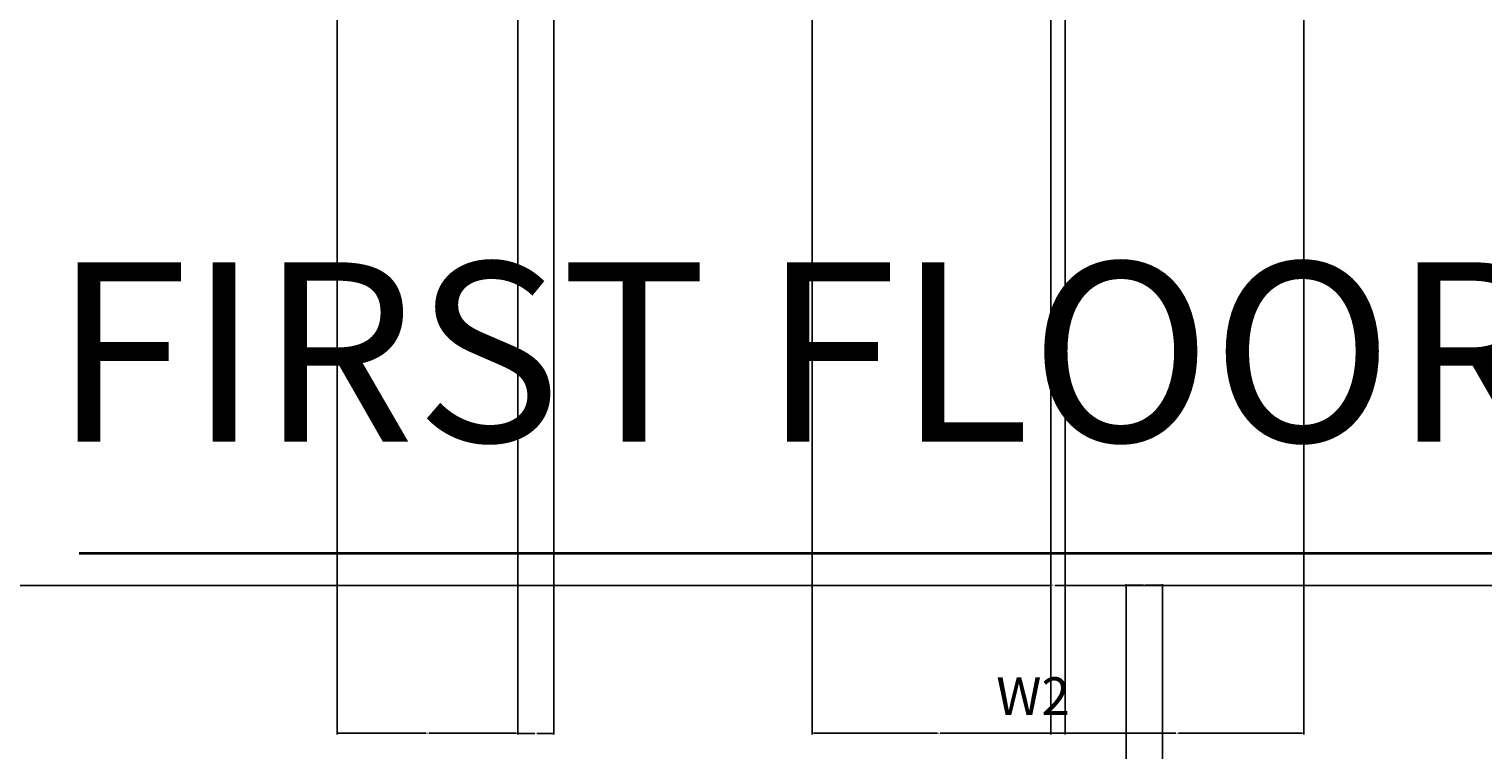
# Model space of a CAD drawing. Units: inches. Extents: x 7359 to 7979, y 33027 to 34263.
# Tile 21 of 32: x 7511 to 7753, y 33630 to 33749. Entities that reach past the tile are written whole.
import ezdxf

# ---------------------------------------------------------------- set-up
doc = ezdxf.new("R2010")
doc.units = ezdxf.units.IN
for name, color, linetype, lineweight in [('A-ANNO-DIMS', 2, 'Continuous', 18), ('A-ANNO-TEXT', 3, 'Continuous', 18), ('A-ANNO-TITL', 7, 'Continuous', 35)]:
    doc.layers.add(name, color=color, linetype=linetype, lineweight=lineweight)
doc.styles.get("Standard").update_dxf_attribs({"font": 'arial.ttf'})
doc.dimstyles.get("Standard").update_dxf_attribs({"dimtxt": 0.18, "dimasz": 0.18, "dimexe": 0.18, "dimexo": 0.0625, "dimgap": 0.09, "dimtad": 0, "dimtih": 1, "dimtoh": 1, "dimdec": 4, "dimzin": 0, "dimdsep": 46, "dimtxsty": 'Standard', "dimcen": 0.09, "dimadec": 0, "dimazin": 0, "dimtfac": 1, "dimtdec": 4, "dimtofl": 0, "dimtmove": 0, "dimatfit": 3, "dimfxl": 1, "dimtolj": 1, "dimtzin": 0, "dimarcsym": 0})

# ---------------------------------------------------------------- blocks, each defined once
blk = doc.blocks.new('*D66')
at = {"layer": 'A-ANNO-DIMS', "color": 0, "lineweight": -2, "transparency": 16777216}
for p, q in [((7468.73, 33627.22), (7468.73, 33657.24)), ((7468.91, 33657.06), (7681.03, 33657.06)), ((7893.95, 33657.06), (7681.82, 33657.06)), ((7894.13, 33627.22), (7894.13, 33657.24))]:
    blk.add_line(p, q, dxfattribs=at)
at = {"layer": 'A-ANNO-DIMS', "color": 0, "transparency": 16777216}
for points in [[(7468.91, 33657.09), (7468.91, 33657.03), (7468.73, 33657.06)], [(7893.95, 33657.09), (7893.95, 33657.03), (7894.13, 33657.06)]]:
    blk.add_solid(points, dxfattribs=at)
at = {"layer": 'Defpoints', "color": 0, "transparency": 16777216}
for p in [(7894.13, 33657.06), (7468.73, 33627.16), (7894.13, 33627.16)]:
    blk.add_point(p, dxfattribs=at)
at = {"layer": 'A-ANNO-DIMS', "color": 0, "transparency": 16777216, "insert": (7681.43, 33657.06), "char_height": 0.18, "attachment_point": 5}
blk.add_mtext('\\A1;425.4', dxfattribs=at)
blk = doc.blocks.new('*D68')
at = {"layer": 'A-ANNO-DIMS', "color": 0, "lineweight": -2, "transparency": 16777216}
for p, q in [((7562.59, 34181.77), (7562.59, 33632.31)), ((7592.59, 34181.77), (7592.59, 33632.31)), ((7562.77, 33632.49), (7577.37, 33632.49)), ((7592.41, 33632.49), (7577.81, 33632.49))]:
    blk.add_line(p, q, dxfattribs=at)
at = {"layer": 'A-ANNO-DIMS', "color": 0, "transparency": 16777216}
for points in [[(7562.77, 33632.52), (7562.77, 33632.46), (7562.59, 33632.49)], [(7592.41, 33632.52), (7592.41, 33632.46), (7592.59, 33632.49)]]:
    blk.add_solid(points, dxfattribs=at)
at = {"layer": 'Defpoints', "color": 0, "transparency": 16777216}
for p in [(7562.59, 34181.83), (7592.59, 34181.83), (7592.59, 33632.49)]:
    blk.add_point(p, dxfattribs=at)
at = {"layer": 'A-ANNO-DIMS', "color": 0, "transparency": 16777216, "insert": (7577.59, 33632.49), "char_height": 0.18, "attachment_point": 5}
blk.add_mtext('\\A1;30', dxfattribs=at)
blk = doc.blocks.new('*D69')
at = {"layer": 'A-ANNO-DIMS', "color": 0, "lineweight": -2, "transparency": 16777216}
for p, q in [((7681.09, 34081.77), (7681.09, 33632.31)), ((7723.09, 34081.77), (7723.09, 33632.31)), ((7681.27, 33632.49), (7701.87, 33632.49)), ((7722.91, 33632.49), (7702.31, 33632.49))]:
    blk.add_line(p, q, dxfattribs=at)
at = {"layer": 'A-ANNO-DIMS', "color": 0, "transparency": 16777216}
for points in [[(7681.27, 33632.52), (7681.27, 33632.46), (7681.09, 33632.49)], [(7722.91, 33632.52), (7722.91, 33632.46), (7723.09, 33632.49)]]:
    blk.add_solid(points, dxfattribs=at)
at = {"layer": 'Defpoints', "color": 0, "transparency": 16777216}
for p in [(7681.09, 34081.83), (7723.09, 34081.83), (7723.09, 33632.49)]:
    blk.add_point(p, dxfattribs=at)
at = {"layer": 'A-ANNO-DIMS', "color": 0, "transparency": 16777216, "insert": (7702.09, 33632.49), "char_height": 0.18, "attachment_point": 5}
blk.add_mtext('\\A1;42', dxfattribs=at)
blk = doc.blocks.new('*D71')
at = {"layer": 'A-ANNO-DIMS', "color": 0, "lineweight": -2, "transparency": 16777216}
for p, q in [((7641.49, 33907.17), (7641.49, 33632.31)), ((7683.49, 33907.17), (7683.49, 33632.31)), ((7641.67, 33632.49), (7662.27, 33632.49)), ((7683.31, 33632.49), (7662.71, 33632.49))]:
    blk.add_line(p, q, dxfattribs=at)
at = {"layer": 'A-ANNO-DIMS', "color": 0, "transparency": 16777216}
for points in [[(7641.67, 33632.52), (7641.67, 33632.46), (7641.49, 33632.49)], [(7683.31, 33632.52), (7683.31, 33632.46), (7683.49, 33632.49)]]:
    blk.add_solid(points, dxfattribs=at)
at = {"layer": 'Defpoints', "color": 0, "transparency": 16777216}
for p in [(7641.49, 33907.23), (7683.49, 33907.23), (7683.49, 33632.49)]:
    blk.add_point(p, dxfattribs=at)
at = {"layer": 'A-ANNO-DIMS', "color": 0, "transparency": 16777216, "insert": (7662.49, 33632.49), "char_height": 0.18, "attachment_point": 5}
blk.add_mtext('\\A1;42', dxfattribs=at)
blk = doc.blocks.new('*D83')
at = {"layer": 'A-ANNO-DIMS', "color": 0, "lineweight": -2, "transparency": 16777216}
for p, q in [((7592.591484, 34081.771428), (7592.591484, 33632.309146)), ((7598.591484, 34081.771428), (7598.591484, 33632.309146)), ((7592.771484, 33632.489146), (7595.442057, 33632.489146)), ((7598.411484, 33632.489146), (7595.740911, 33632.489146))]:
    blk.add_line(p, q, dxfattribs=at)
at = {"layer": 'A-ANNO-DIMS', "color": 0, "transparency": 16777216}
for points in [[(7592.771484, 33632.519146), (7592.771484, 33632.459146), (7592.591484, 33632.489146)], [(7598.411484, 33632.519146), (7598.411484, 33632.459146), (7598.591484, 33632.489146)]]:
    blk.add_solid(points, dxfattribs=at)
at = {"layer": 'Defpoints', "color": 0, "transparency": 16777216}
for p in [(7592.591484, 34081.833928), (7598.591484, 34081.833928), (7598.591484, 33632.489146)]:
    blk.add_point(p, dxfattribs=at)
at = {"layer": 'A-ANNO-DIMS', "color": 0, "transparency": 16777216, "insert": (7595.591484, 33632.489146), "char_height": 0.18, "attachment_point": 5}
blk.add_mtext('\\A1;6', dxfattribs=at)
blk = doc.blocks.new('*D89')
at = {"layer": 'A-ANNO-DIMS', "color": 0, "lineweight": -2, "transparency": 16777216}
for p, q in [((7693.626578, 33301.124789), (7693.626578, 33657.242289)), ((7693.806578, 33657.062289), (7696.477151, 33657.062289)), ((7699.446578, 33657.062289), (7696.776005, 33657.062289)), ((7699.626578, 33301.124789), (7699.626578, 33657.242289))]:
    blk.add_line(p, q, dxfattribs=at)
at = {"layer": 'A-ANNO-DIMS', "color": 0, "transparency": 16777216}
for points in [[(7693.806578, 33657.092289), (7693.806578, 33657.032289), (7693.626578, 33657.062289)], [(7699.446578, 33657.092289), (7699.446578, 33657.032289), (7699.626578, 33657.062289)]]:
    blk.add_solid(points, dxfattribs=at)
at = {"layer": 'Defpoints', "color": 0, "transparency": 16777216}
for p in [(7699.626578, 33657.062289), (7693.626578, 33301.062289), (7699.626578, 33301.062289)]:
    blk.add_point(p, dxfattribs=at)
at = {"layer": 'A-ANNO-DIMS', "color": 0, "transparency": 16777216, "insert": (7696.626578, 33657.062289), "char_height": 0.18, "attachment_point": 5}
blk.add_mtext('\\A1;6', dxfattribs=at)

msp = doc.modelspace()

# ---------------------------------------------------------------- linework, layer by layer
at = {"layer": 'A-ANNO-TITL'}
msp.add_line((7519.7539, 33662.3891), (7797.0359, 33662.3891), dxfattribs=at)

# ---------------------------------------------------------------- texts
at = {"layer": 'A-ANNO-TEXT'}
msp.add_text('W2', height=6.25941, dxfattribs=at).set_placement((7672.043, 33635.5363))
at = {"layer": 'A-ANNO-TITL'}
msp.add_text('FIRST FLOOR', height=29.769676, dxfattribs=at).set_placement((7515.4376, 33680.9181))

# ---------------------------------------------------------------- dimensions: what is measured, and where the dimension line sits
at = {"layer": 'A-ANNO-DIMS'}
for base, p1, p2, override, picture, middle in [((7592.5915, 33632.4891), (7562.5915, 34181.8339), (7592.5915, 34181.8339), {"dimdec": 0, "dimlfac": 1, "dimrnd": 0, "dimzin": 0, "dimdsep": 46, "dimlunit": 2}, '*D68', (7577.5915, 33632.4891)), ((7598.5915, 33632.4891), (7592.5915, 34081.8339), (7598.5915, 34081.8339), {"dimdec": 0, "dimlfac": 1, "dimrnd": 0, "dimzin": 0, "dimdsep": 46, "dimlunit": 2}, '*D83', (7595.5915, 33632.4891)), ((7723.0915, 33632.4891), (7681.0915, 34081.8339), (7723.0915, 34081.8339), {"dimdec": 0, "dimlfac": 1, "dimrnd": 0, "dimzin": 0, "dimdsep": 46, "dimlunit": 2}, '*D69', (7702.0915, 33632.4891)), ((7683.4915, 33632.4891), (7641.4915, 33907.2339), (7683.4915, 33907.2339), {"dimdec": 0, "dimlfac": 1, "dimrnd": 0, "dimzin": 0, "dimdsep": 46, "dimlunit": 2}, '*D71', (7662.4915, 33632.4891)), ((7894.1266, 33657.0623), (7468.7266, 33627.1623), (7894.1266, 33627.1623), {"dimdec": 1, "dimlfac": 1, "dimrnd": 0, "dimzin": 0, "dimdsep": 46, "dimlunit": 2}, '*D66', (7681.4266, 33657.0623)), ((7699.6266, 33657.0623), (7693.6266, 33301.0623), (7699.6266, 33301.0623), {"dimdec": 0, "dimlfac": 1, "dimrnd": 0, "dimzin": 0, "dimdsep": 46, "dimlunit": 2}, '*D89', (7696.6266, 33657.0623))]:
    dim = msp.add_linear_dim(base=base, p1=p1, p2=p2, dimstyle='Standard', override=override, dxfattribs=at)
    dim.commit()
    dim.dimension.update_dxf_attribs({"geometry": picture, "text_midpoint": middle})

doc.saveas('drawing.dxf')
